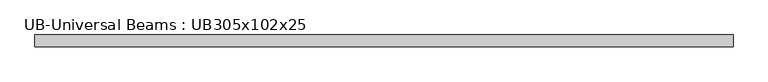
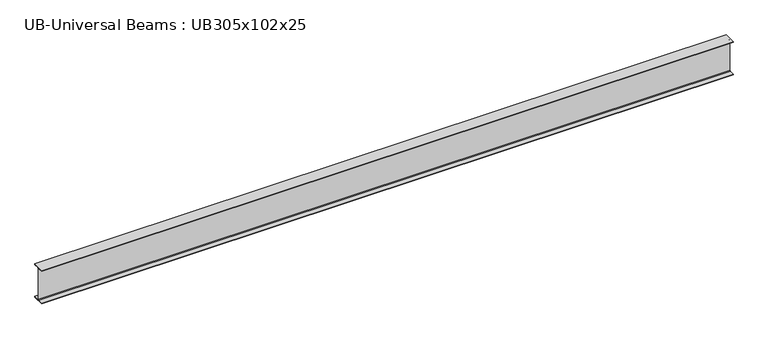
"""IFC4 building model written with IfcOpenShell, lengths in millimetres: beam geometry, UB-Universal Beams : UB305x102x25."""

from ifc_helpers import new_model, si_unit, point, frame, frame_2d, origin, place, context, project, spatial, polyline, circle_curve, trimmed, segment, composite_curve, outline, extrude, source, transform, mapped, element, save


def ub_universal_beams_ub305x102x25_07ba02ff(model_context):
    return source(origin(), model_context, "Body", "SweptSolid", [
        extrude(outline(composite_curve([segment(polyline([(50.8, -145.55), (50.8, -152.55), (-50.8, -152.55), (-50.8, -145.55), (-10.5, -145.55)]), True, "CONTINUOUS"), segment(trimmed(circle_curve(frame_2d((-10.5, -137.95)), 7.6), [point((-10.5, -145.55))], [point((-2.9, -137.95))], True, "CARTESIAN"), True, "CONTINUOUS"), segment(polyline([(-2.9, -137.95), (-2.9, 137.95)]), True, "CONTINUOUS"), segment(trimmed(circle_curve(frame_2d((-10.5, 137.95)), 7.6), [point((-2.9, 137.95))], [point((-10.5, 145.55))], True, "CARTESIAN"), True, "CONTINUOUS"), segment(polyline([(-10.5, 145.55), (-50.8, 145.55), (-50.8, 152.55), (50.8, 152.55), (50.8, 145.55), (10.5, 145.55)]), True, "CONTINUOUS"), segment(trimmed(circle_curve(frame_2d((10.5, 137.95)), 7.6), [point((10.5, 145.55))], [point((2.9, 137.95))], True, "CARTESIAN"), True, "CONTINUOUS"), segment(polyline([(2.9, 137.95), (2.9, -137.95)]), True, "CONTINUOUS"), segment(trimmed(circle_curve(frame_2d((10.5, -137.95)), 7.6), [point((2.9, -137.95))], [point((10.5, -145.55))], True, "CARTESIAN"), True, "CONTINUOUS"), segment(polyline([(10.5, -145.55), (50.8, -145.55)]), True, "CONTINUOUS")], self_intersect=False)), frame((-3000.0, 0.0, 0.0), z_axis=(1.0, 0.0, 0.0), x_axis=(0.0, 1.0, 0.0)), (0.0, 0.0, 1.0), 6000.0),
    ])


if __name__ == "__main__":
    model = new_model("IFC4")
    model_context = context("Model", 3, world=origin())
    ifc_project = project(units=[si_unit("LENGTHUNIT", "METRE", prefix="MILLI")], contexts=[model_context])
    site = spatial("IfcSite", under=ifc_project)
    building = spatial("IfcBuilding", under=site)
    placement = place(None, origin())
    ub_universal_beams_ub305x102x25_shape = ub_universal_beams_ub305x102x25_07ba02ff(model_context)
    element("IfcBeam", 1, ObjectType="UB-Universal Beams : UB305x102x25", at=placement, inside=building, context=model_context, shape_type="MappedRepresentation", body=[
        mapped(ub_universal_beams_ub305x102x25_shape, transform((0.0, 0.0, 0.0), x_axis=(1.0, 0.0, 0.0), y_axis=(0.0, 1.0, 0.0), z_axis=(0.0, 0.0, 1.0))),
    ])
    save(model, "model.ifc")

# Revit data of these elements
# Type "UB-Universal Beams : UB305x102x25"
#   Section Name Key = "UB305X102X25"
#   Width = 10.16 cm
#   Web Thickness = 0.58 cm
#   Web Fillet = 0.76 cm
#   Warping Constant = 27300.0 cm⁶
#   Torsional Moment of Inertia = 4.77 cm⁴
#   Section Area = 31.6 cm²
#   Plastic Modulus weak axis = 39.0 cm³
#   Plastic Modulus strong axis = 342.0 cm³
#   Nominal Weight = 24.7999 kgf/m
#   Moment of Inertia weak axis = 123.00 cm⁴
#   Moment of Inertia strong axis = 4455.00 cm⁴
#   Height = 30.51 cm
#   Flange Thickness = 0.7 cm
#   Elastic Modulus weak axis = 24.2 cm³
#   Elastic Modulus strong axis = 292.0 cm³
#   Centroid Vertical = 15.255 cm
#   Centroid Horizontal = 5.08 cm
#   Bolt Spacing = 5.4 cm
#   Length [instance default] = 1.5 m
#   Structural Material [instance default] = Metal - Steel 43-275
#   Type Comments = ""
#   Assembly Code = ""
# Element 1 (IfcBeam, "UB-Universal Beams : UB305x102x25")
#   Materials on its faces: "Metal - Steel 43-275"
# Materials
#   "Metal - Steel 43-275": class "Metal", colour RGB 247 247 247, transparency 0, Cost = 0
